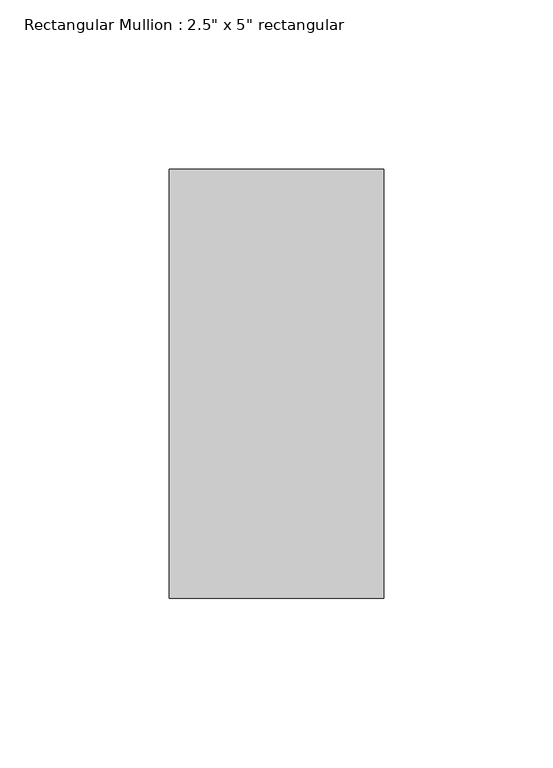
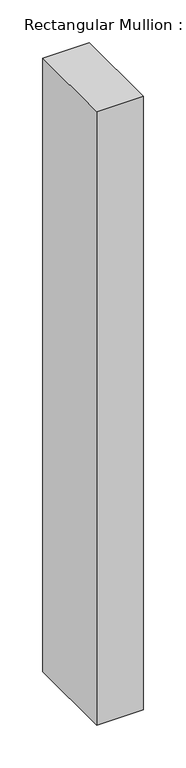
"""IFC4 building model written with IfcOpenShell, lengths in millimetres: member geometry."""

from ifc_helpers import new_model, si_unit, frame, origin, place, context, project, spatial, polyline, outline, extrude, source, transform, mapped, element, save


def member_3ee5b9af(model_context):
    return source(origin(), model_context, "Body", "SweptSolid", [
        extrude(outline(polyline([(0.0, 63.5), (0.0, -63.5), (-63.5, -63.5), (-63.5, 63.5), (0.0, 63.5)])), frame((0.0, 0.0, -880.2652244), z_axis=(0.0, 0.0, 1.0), x_axis=(1.0, 0.0, 0.0)), (0.0, 0.0, 1.0), 880.2652244),
    ])


if __name__ == "__main__":
    model = new_model("IFC4")
    model_context = context("Model", 3, world=origin())
    ifc_project = project(units=[si_unit("LENGTHUNIT", "METRE", prefix="MILLI")], contexts=[model_context])
    site = spatial("IfcSite", under=ifc_project)
    building = spatial("IfcBuilding", under=site)
    placement = place(None, origin())
    member_shape = member_3ee5b9af(model_context)
    element("IfcMember", 1, ObjectType="Rectangular Mullion : 2.5\" x 5\" rectangular", at=placement, inside=building, context=model_context, shape_type="MappedRepresentation", body=[
        mapped(member_shape, transform((0.0, 0.0, 0.0), x_axis=(1.0, 0.0, 0.0), y_axis=(0.0, 1.0, 0.0), z_axis=(0.0, 0.0, 1.0))),
    ])
    save(model, "model.ifc")

# Revit data of these elements
# Type "Rectangular Mullion : 2.5\" x 5\" rectangular"
#   built-in parameter 1007304 = 0.416667 (stored number, unit not read)
#   built-in parameter 1007301 = 0.104167 (stored number, unit not read)
#   built-in parameter 1007300 = 0.104167 (stored number, unit not read)
# Element 1 (IfcMember, "Rectangular Mullion : 2.5\" x 5\" rectangular")
#   Materials on its faces: "Aluminum"
# Materials
#   "Aluminum": class "Metal", colour RGB 247 247 247, transparency 0, Description = "Aluminum 6061", Cost = 0
